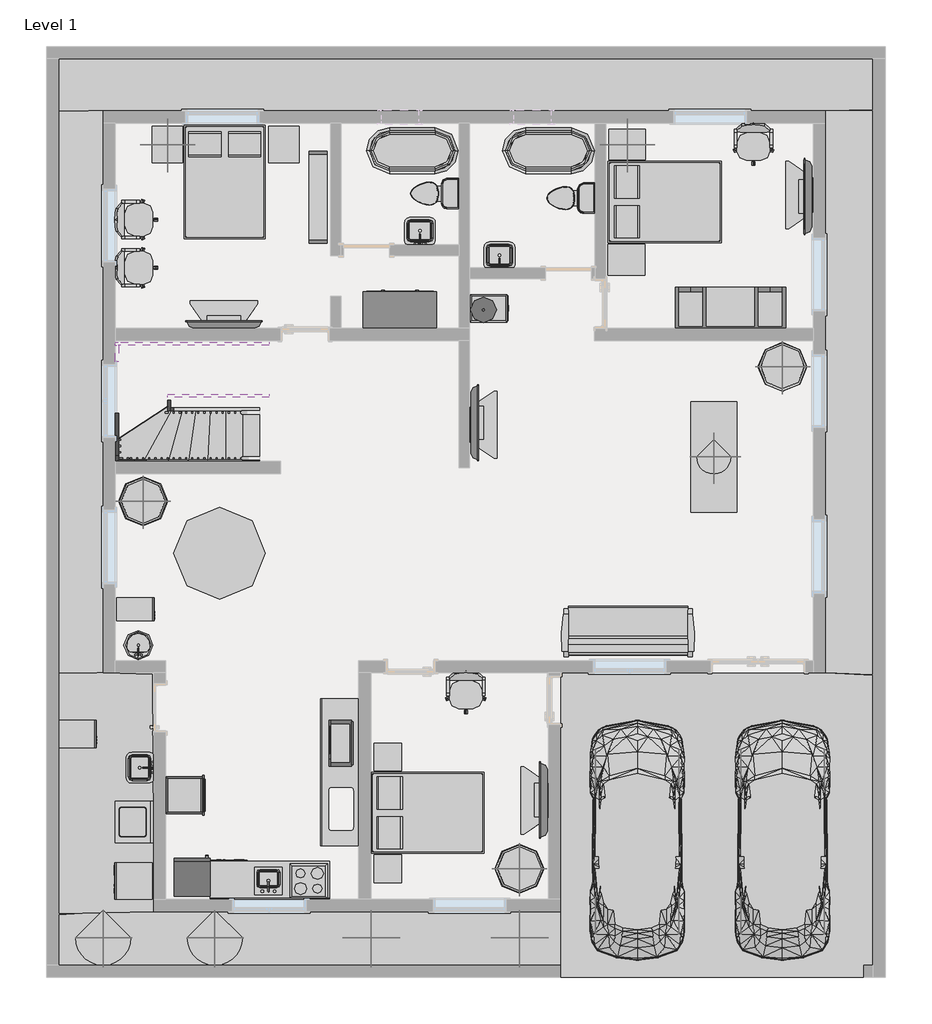
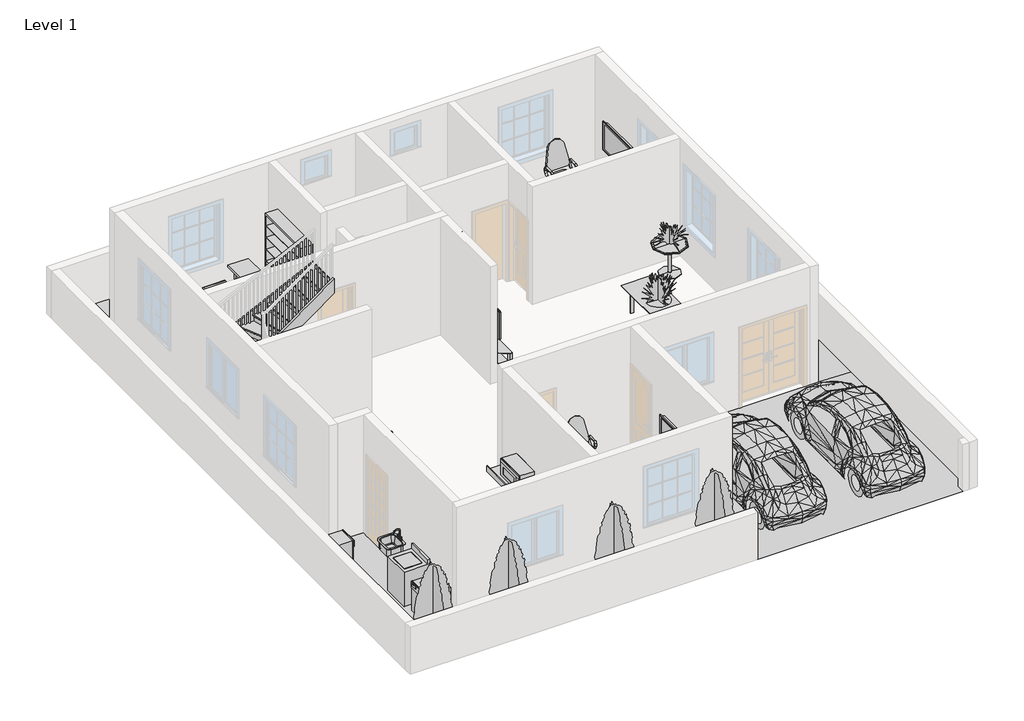
# One storey, part 3 of 3: 33 furniture elements, 18 proxies, 10 flow terminals, 10 geographic elements, 9 members, 1 stair flight.
# Revit data of these elements (continued)
# Materials (continued)
#   "Laminate, Linen, Matte": class "Plastic", colour RGB 249 239 230, transparency 0, Description = "Plastic Laminate - Linen, Matte", Cost = 0
#   "Porcelain, Ivory": class "Ceramic", colour RGB 247 247 239, transparency 0, Description = "Porcelain, ivory", Cost = 0
#   "Birch": class "Wood", colour RGB 224 178 126, transparency 0, Description = "Betula Alleghaniensis", Cost = 0
#   "Linen, White": class "Textile", colour RGB 247 247 239, transparency 0, Description = "Linen, white", Cost = 0
#   "Textile - Slate Blue": class "Fabric", colour RGB 98 102 118, transparency 0
#   "Laminate - Ivory, Glossy": colour RGB 247 247 239, transparency 0
#   "Cherry": class "Wood", colour RGB 226 177 128, transparency 0, Description = "Prunus Serotina", Cost = 0
#   "Linen, Beige": class "Textile", colour RGB 249 239 230, transparency 0, Description = "Linen, beige", Cost = 0
#   "Melamine - Gray": class "Wood", colour RGB 49 49 49, transparency 0
#   "Glass - Clear, Grey": class "Glass", colour RGB 252 255 255, transparency 0.64
#   "Pine": class "Wood", colour RGB 223 192 134, transparency 0, Description = "Pinus Echinata", Cost = 0
#   "Default Mass Floor": colour RGB 0 255 0, transparency 0, Cost = 0
#   "Glass": class "Glass", colour RGB 0 128 192, transparency 0.75, Description = "Soda Lime Glass", Cost = 0
#   "Steel": class "Metal", colour RGB 247 247 247, transparency 0, Description = "Steel, mill finish", Cost = 0
#   "Cabinets - Panel/Glass": colour RGB 252 255 255, transparency 0.72
#   "Counter Top": class "Wood", colour RGB 226 177 128, transparency 0
#   "TV - Black": colour RGB 49 49 49, transparency 0
#   "TV - Glass": colour RGB 157 157 157, transparency 0.9
#   "TV - Screen": colour RGB 0 0 0, transparency 0
#   "Glass - Shelves": class "Glass", colour RGB 167 167 167, transparency 0.9
